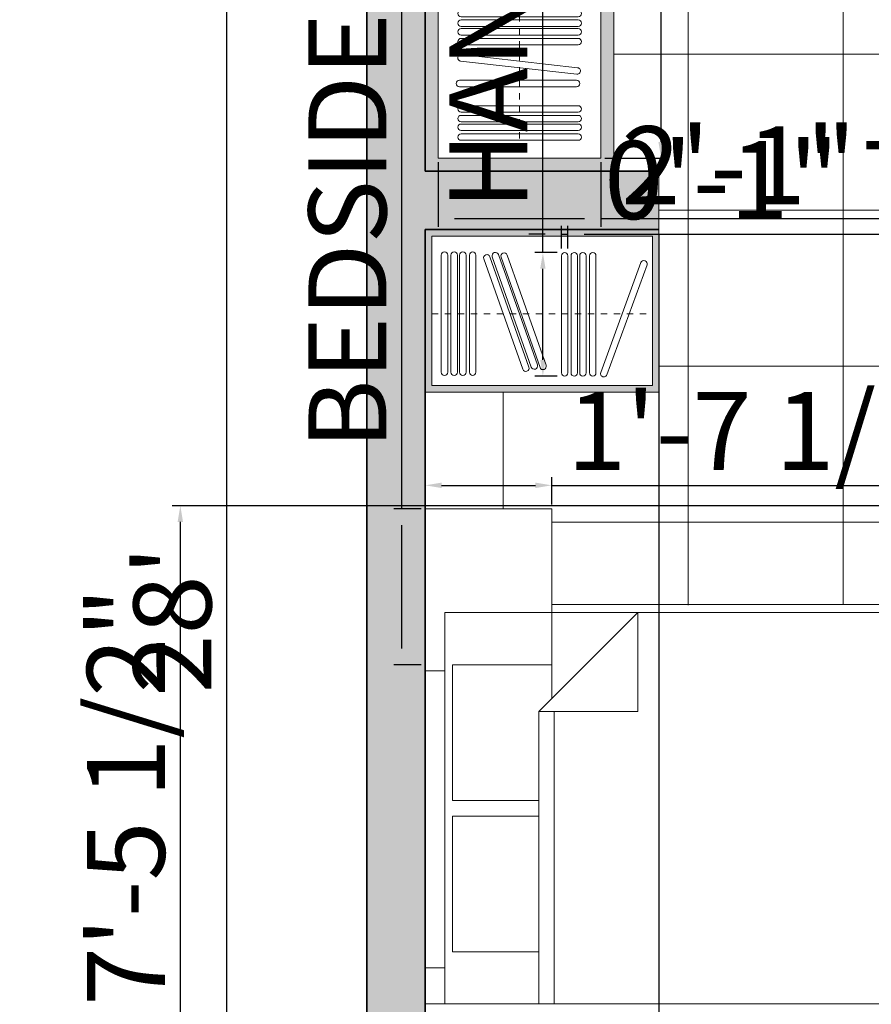
# Model space of a CAD drawing. Units: millimetres. Extents: x 542930 to 543750, y 628093 to 628738.
# Tile 3 of 14: x 542930 to 543061, y 628363 to 628514. Entities that reach past the tile are written whole.
import ezdxf

# ---------------------------------------------------------------- set-up
doc = ezdxf.new("R2010")
doc.units = ezdxf.units.MM
doc.linetypes.add('JIS_02_1.0', pattern=[2, 1, -1])
for name, color, linetype, lineweight in [('A-ANNO-DIMS', 2, 'Continuous', 18), ('A-FURN', 8, 'Continuous', 18), ('A-FURN-MILL', 8, 'Continuous', 18), ('A-FURN-MILL-HIDN', 8, 'JIS_02_1.0', 13), ('A-FURN-PATT', 9, 'Continuous', 13), ('A-WALL', 7, 'Continuous', 35)]:
    doc.layers.add(name, color=color, linetype=linetype, lineweight=lineweight)
doc.layers.add('A-FLOR-PATT', color=241, linetype='Continuous', lineweight=13, true_color=0xf7abae)
doc.layers.add('A-WALL-PATT', color=251, linetype='Continuous', lineweight=13, true_color=0x636466)
doc.styles.get("Standard").update_dxf_attribs({"font": 'arial.ttf'})
doc.dimstyles.new('ISO-25', dxfattribs={"dimtxt": 12, "dimasz": 2.5, "dimexe": 1.25, "dimexo": 0.625, "dimtad": 1, "dimdec": 0, "dimlunit": 3, "dimtxsty": 'Standard', "dimcen": 2.5, "dimadec": 0, "dimazin": 0, "dimtfac": 1, "dimtdec": 0, "dimtmove": 0, "dimatfit": 3, "dimfxl": 1, "dimarcsym": 0})

# ---------------------------------------------------------------- blocks, each defined once
blk = doc.blocks.new('Bed - Queen')
for p, q in [((0, -80.00003), (0, 0)), ((0, 0), (59.99999, 0)), ((59.99999, 0), (59.99999, -80.00003)), ((7.99999, -1.2), (28.79998, -1.2)), ((7.99999, -14.4), (7.99999, -1.2)), ((28.79998, -1.2), (28.79998, -14.4)), ((31.19999, -1.2), (51.99999, -1.2)), ((31.19999, -14.4), (31.19999, -1.2)), ((51.99999, -1.2), (51.99999, -16.4)), ((0, -14.4), (44.8, -14.4)), ((59.99999, -29.6), (44.8, -14.4)), ((44.8, -14.4), (44.8, -29.6)), ((51.99999, -16.4), (46.79936, -16.4)), ((44.8, -16.8), (0, -16.8)), ((44.8, -29.6), (59.99999, -29.6)), ((59.99999, -80.00003), (0, -80.00003))]:
    blk.add_line(p, q)
blk = doc.blocks.new('*D20')
at = {"layer": 'A-ANNO-DIMS', "color": 0, "lineweight": -2, "transparency": 16777216}
for p, q in [((542983.04, 628589.83), (542960.8, 628589.83)), ((542962.05, 628587.33), (542962.05, 628256.33)), ((542983.04, 628253.83), (542960.8, 628253.83))]:
    blk.add_line(p, q, dxfattribs=at)
at = {"layer": 'A-ANNO-DIMS', "color": 0, "transparency": 16777216}
for points in [[(542961.64, 628587.33), (542962.47, 628587.33), (542962.05, 628589.83)], [(542961.64, 628256.33), (542962.47, 628256.33), (542962.05, 628253.83)]]:
    blk.add_solid(points, dxfattribs=at)
at = {"layer": 'Defpoints', "color": 0, "transparency": 16777216}
for p in [(542983.67, 628589.83), (542962.05, 628253.83), (542983.67, 628253.83)]:
    blk.add_point(p, dxfattribs=at)
at = {"layer": 'A-ANNO-DIMS', "color": 0, "transparency": 16777216, "insert": (542955.3, 628421.83), "char_height": 12, "attachment_point": 5, "rotation": 90}
blk.add_mtext("28'", dxfattribs=at)
blk = doc.blocks.new('WARDROBE-DRESS-RAIL')
for p, q in [((0, 0), (0, 62)), ((0, 62), (25, 62)), ((3.52, 60.83), (21.52, 60.83)), ((25, 0), (25, 62)), ((3.52, 59.83), (21.52, 59.83)), ((3.52, 59.35), (21.52, 59.35)), ((3.52, 58.35), (21.52, 58.35)), ((3.52, 58.02), (21.52, 58.02)), ((3.52, 57.02), (21.52, 57.02)), ((3.52, 56.51), (21.52, 56.51)), ((3.52, 55.51), (21.52, 55.51)), ((3.57, 51.08), (21.23, 54.55)), ((3.76, 50.1), (21.43, 53.57)), ((3.52, 49.31), (21.52, 49.31)), ((3.52, 48.31), (21.52, 48.31)), ((3.52, 47.82), (21.52, 47.82)), ((3.52, 46.82), (21.52, 46.82)), ((3.52, 46.49), (21.52, 46.49)), ((3.52, 45.49), (21.52, 45.49)), ((3.57, 41.35), (21.23, 44.82)), ((3.57, 39.47), (21.23, 42.94)), ((3.76, 40.37), (21.43, 43.84)), ((3.76, 38.49), (21.43, 41.96)), ((3.52, 35.91), (21.52, 35.91)), ((3.52, 34.91), (21.52, 34.91)), ((3.52, 34.43), (21.52, 34.43)), ((3.52, 33.43), (21.52, 33.43)), ((3.52, 33.1), (21.52, 33.1)), ((3.52, 32.1), (21.52, 32.1)), ((3.52, 31.59), (21.52, 31.59)), ((3.52, 30.59), (21.52, 30.59)), ((3.27, 26.51), (21.27, 26.51)), ((3.27, 25.51), (21.27, 25.51)), ((3.52, 22.74), (21.52, 22.74)), ((3.52, 21.74), (21.52, 21.74)), ((3.52, 21.26), (21.52, 21.26)), ((3.52, 20.26), (21.52, 20.26)), ((3.52, 19.93), (21.52, 19.93)), ((3.52, 18.93), (21.52, 18.93)), ((3.52, 18.42), (21.52, 18.42)), ((3.52, 17.42), (21.52, 17.42)), ((3.56, 15.93), (21.44, 13.91)), ((3.44, 14.93), (21.33, 12.92)), ((3.27, 11.99), (21.27, 11.99)), ((3.27, 10.99), (21.27, 10.99)), ((3.52, 8.06), (21.52, 8.06)), ((3.52, 7.06), (21.52, 7.06)), ((3.52, 6.58), (21.52, 6.58)), ((3.52, 5.58), (21.52, 5.58)), ((3.52, 5.25), (21.52, 5.25)), ((3.52, 4.25), (21.52, 4.25)), ((3.52, 3.74), (21.52, 3.74)), ((3.52, 2.74), (21.52, 2.74)), ((0, 0), (25, 0))]:
    blk.add_line(p, q)
for centre, start, end in [((3.52, 60.33), 90, 270), ((21.52, 60.33), 270, 90), ((3.52, 58.85), 90, 270), ((21.52, 58.85), 270, 90), ((3.52, 57.52), 90, 270), ((21.52, 57.52), 270, 90), ((3.52, 56.01), 90, 270), ((21.52, 56.01), 270, 90), ((21.33, 54.06), 281.1082, 101.1082), ((3.67, 50.59), 101.1082, 281.1082), ((3.52, 48.81), 90, 270), ((21.52, 48.81), 270, 90), ((3.52, 47.32), 90, 270), ((21.52, 47.32), 270, 90), ((3.52, 45.99), 90, 270), ((21.52, 45.99), 270, 90), ((21.33, 44.33), 281.1082, 101.1082), ((21.33, 42.45), 281.1082, 101.1082), ((3.67, 40.86), 101.1082, 281.1082), ((3.67, 38.98), 101.1082, 281.1082), ((3.52, 35.41), 90, 270), ((21.52, 35.41), 270, 90), ((3.52, 33.93), 90, 270), ((21.52, 33.93), 270, 90), ((3.52, 32.6), 90, 270), ((21.52, 32.6), 270, 90), ((3.52, 31.09), 90, 270), ((21.52, 31.09), 270, 90), ((3.27, 26.01), 90, 270), ((21.27, 26.01), 270, 90), ((3.52, 22.24), 90, 270), ((21.52, 22.24), 270, 90), ((3.52, 20.76), 90, 270), ((21.52, 20.76), 270, 90), ((3.52, 19.43), 90, 270), ((21.52, 19.43), 270, 90), ((3.52, 17.92), 90, 270), ((21.52, 17.92), 270, 90), ((3.5, 15.43), 83.5593, 263.5593), ((21.39, 13.41), 263.5593, 83.5611), ((3.27, 11.49), 90, 270), ((21.27, 11.49), 270, 90), ((3.52, 7.56), 90, 270), ((21.52, 7.56), 270, 90), ((3.52, 6.08), 90, 270), ((21.52, 6.08), 270, 90), ((3.52, 4.75), 90, 270), ((21.52, 4.75), 270, 90), ((3.52, 3.24), 90, 270), ((21.52, 3.24), 270, 90)]:
    blk.add_arc(centre, 0.5, start, end)
blk = doc.blocks.new('WARDROBE-HANGER')
for p, q in [((0, 0.5), (0, 18.5)), ((1, 0.5), (1, 18.5))]:
    blk.add_line(p, q)
for centre, start, end in [((0.5, 18.5), 0, 180), ((0.5, 0.5), 180, 0)]:
    blk.add_arc(centre, 0.5, start, end)
blk = doc.blocks.new('BED-SIDE-STAND')
for p, q in [((19.46, 24), (0, 24)), ((19.46, 0), (19.46, 24))]:
    blk.add_line(p, q)
blk = doc.blocks.new('*D31')
at = {"layer": 'A-ANNO-DIMS', "color": 0, "lineweight": -2, "transparency": 16777216}
for p, q in [((543010.77, 628478.3), (543010.77, 628630.92)), ((543012.99, 628478.3), (543009.52, 628478.3)), ((543010.77, 628461.8), (543010.77, 628475.8)), ((543012.99, 628459.3), (543009.52, 628459.3))]:
    blk.add_line(p, q, dxfattribs=at)
at = {"layer": 'A-ANNO-DIMS', "color": 0, "transparency": 16777216}
for points in [[(543010.35, 628475.8), (543011.18, 628475.8), (543010.77, 628478.3)], [(543010.35, 628461.8), (543011.18, 628461.8), (543010.77, 628459.3)]]:
    blk.add_solid(points, dxfattribs=at)
at = {"layer": 'Defpoints', "color": 0, "transparency": 16777216}
for p in [(543010.77, 628478.3), (543013.62, 628478.3), (543013.62, 628459.3)]:
    blk.add_point(p, dxfattribs=at)
at = {"layer": 'A-ANNO-DIMS', "color": 0, "transparency": 16777216, "insert": (543003.94, 628555.86), "char_height": 12, "attachment_point": 5, "rotation": 90}
blk.add_mtext('HANGER 1\'-7" TYP.', dxfattribs=at)
blk = doc.blocks.new('*D32')
at = {"layer": 'A-ANNO-DIMS', "color": 0, "lineweight": -2, "transparency": 16777216}
for p, q in [((543011.12, 628481.15), (543008.62, 628481.15)), ((543013.62, 628478.92), (543013.62, 628482.4)), ((543013.62, 628481.15), (543014.62, 628481.15)), ((543014.62, 628478.92), (543014.62, 628482.4)), ((543017.12, 628481.15), (543094.01, 628481.15))]:
    blk.add_line(p, q, dxfattribs=at)
at = {"layer": 'A-ANNO-DIMS', "color": 0, "transparency": 16777216}
for points in [[(543011.12, 628481.56), (543011.12, 628480.73), (543013.62, 628481.15)], [(543017.12, 628481.56), (543017.12, 628480.73), (543014.62, 628481.15)]]:
    blk.add_solid(points, dxfattribs=at)
at = {"layer": 'Defpoints', "color": 0, "transparency": 16777216}
for p in [(543014.62, 628481.15), (543013.62, 628478.3), (543014.62, 628478.3)]:
    blk.add_point(p, dxfattribs=at)
at = {"layer": 'A-ANNO-DIMS', "color": 0, "transparency": 16777216, "insert": (543056.82, 628487.9), "char_height": 12, "attachment_point": 5}
blk.add_mtext('0\'-1" TYP.', dxfattribs=at)
blk = doc.blocks.new('*D43')
at = {"layer": 'A-ANNO-DIMS', "color": 0, "lineweight": -2, "transparency": 16777216}
for p, q in [((543028.97, 628554.83), (543028.97, 628735.47)), ((543020.29, 628554.83), (543030.22, 628554.83)), ((543028.97, 628495.33), (543028.97, 628552.33)), ((543020.29, 628492.83), (543030.22, 628492.83))]:
    blk.add_line(p, q, dxfattribs=at)
at = {"layer": 'A-ANNO-DIMS', "color": 0, "transparency": 16777216}
for points in [[(543028.55, 628552.33), (543029.38, 628552.33), (543028.97, 628554.83)], [(543028.55, 628495.33), (543029.38, 628495.33), (543028.97, 628492.83)]]:
    blk.add_solid(points, dxfattribs=at)
at = {"layer": 'Defpoints', "color": 0, "transparency": 16777216}
for p in [(543019.67, 628554.83), (543028.97, 628554.83), (543019.67, 628492.83)]:
    blk.add_point(p, dxfattribs=at)
at = {"layer": 'A-ANNO-DIMS', "color": 0, "transparency": 16777216, "insert": (543022.14, 628646.4), "char_height": 12, "attachment_point": 5, "rotation": 90}
blk.add_mtext('DRESS RAIL 5\'-2" TYP.', dxfattribs=at)
blk = doc.blocks.new('*D44')
at = {"layer": 'A-ANNO-DIMS', "color": 0, "lineweight": -2, "transparency": 16777216}
for p, q in [((542994.67, 628492.2), (542994.67, 628482.28)), ((543019.67, 628492.2), (543019.67, 628482.28)), ((542997.17, 628483.53), (543017.17, 628483.53)), ((543019.67, 628483.53), (543096.77, 628483.53))]:
    blk.add_line(p, q, dxfattribs=at)
at = {"layer": 'A-ANNO-DIMS', "color": 0, "transparency": 16777216}
for points in [[(542997.17, 628483.94), (542997.17, 628483.11), (542994.67, 628483.53)], [(543017.17, 628483.94), (543017.17, 628483.11), (543019.67, 628483.53)]]:
    blk.add_solid(points, dxfattribs=at)
at = {"layer": 'Defpoints', "color": 0, "transparency": 16777216}
for p in [(542994.67, 628492.83), (543019.67, 628492.83), (543019.67, 628483.53)]:
    blk.add_point(p, dxfattribs=at)
at = {"layer": 'A-ANNO-DIMS', "color": 0, "transparency": 16777216, "insert": (543059.47, 628490.18), "char_height": 12, "attachment_point": 5}
blk.add_mtext('2\'-1" TYP.', dxfattribs=at)
blk = doc.blocks.new('*D59')
at = {"layer": 'A-ANNO-DIMS', "color": 0, "lineweight": -2, "transparency": 16777216}
for p, q in [((542989.07, 628438.89), (542989.07, 628654.99)), ((542992.04, 628438.89), (542987.82, 628438.89)), ((542989.07, 628417.39), (542989.07, 628436.39)), ((542992.04, 628414.89), (542987.82, 628414.89))]:
    blk.add_line(p, q, dxfattribs=at)
at = {"layer": 'A-ANNO-DIMS', "color": 0, "transparency": 16777216}
for points in [[(542988.65, 628436.39), (542989.48, 628436.39), (542989.07, 628438.89)], [(542988.65, 628417.39), (542989.48, 628417.39), (542989.07, 628414.89)]]:
    blk.add_solid(points, dxfattribs=at)
at = {"layer": 'Defpoints', "color": 0, "transparency": 16777216}
for p in [(542989.07, 628438.89), (542992.67, 628438.89), (542992.67, 628414.89)]:
    blk.add_point(p, dxfattribs=at)
at = {"layer": 'A-ANNO-DIMS', "color": 0, "transparency": 16777216, "insert": (542982.24, 628548.19), "char_height": 12, "attachment_point": 5, "rotation": 90}
blk.add_mtext('BEDSIDE STAND 2\'-0" TYP.', dxfattribs=at)
blk = doc.blocks.new('*D60')
at = {"layer": 'A-ANNO-DIMS', "color": 0, "lineweight": -2, "transparency": 16777216}
for p, q in [((542992.67, 628439.52), (542992.67, 628443.74)), ((543012.12, 628439.52), (543012.12, 628443.74)), ((542995.17, 628442.49), (543009.62, 628442.49)), ((543012.12, 628442.49), (543115.85, 628442.49))]:
    blk.add_line(p, q, dxfattribs=at)
at = {"layer": 'A-ANNO-DIMS', "color": 0, "transparency": 16777216}
for points in [[(542995.17, 628442.91), (542995.17, 628442.08), (542992.67, 628442.49)], [(543009.62, 628442.91), (543009.62, 628442.08), (543012.12, 628442.49)]]:
    blk.add_solid(points, dxfattribs=at)
at = {"layer": 'Defpoints', "color": 0, "transparency": 16777216}
for p in [(543012.12, 628442.49), (542992.67, 628438.89), (543012.12, 628438.89)]:
    blk.add_point(p, dxfattribs=at)
at = {"layer": 'A-ANNO-DIMS', "color": 0, "transparency": 16777216, "insert": (543065.24, 628449.32), "char_height": 12, "attachment_point": 5}
blk.add_mtext('1\'-7 1/2" TYP.', dxfattribs=at)
blk = doc.blocks.new('*D75')
at = {"layer": 'A-ANNO-DIMS', "color": 0, "lineweight": -2, "transparency": 16777216}
for p, q in [((543324.54, 628439.36), (542953.72, 628439.36)), ((542954.97, 628352.33), (542954.97, 628436.86)), ((543324.54, 628349.83), (542953.72, 628349.83))]:
    blk.add_line(p, q, dxfattribs=at)
at = {"layer": 'A-ANNO-DIMS', "color": 0, "transparency": 16777216}
for points in [[(542954.55, 628436.86), (542955.38, 628436.86), (542954.97, 628439.36)], [(542954.55, 628352.33), (542955.38, 628352.33), (542954.97, 628349.83)]]:
    blk.add_solid(points, dxfattribs=at)
at = {"layer": 'Defpoints', "color": 0, "transparency": 16777216}
for p in [(542954.97, 628439.36), (543325.17, 628439.36), (543325.17, 628349.83)]:
    blk.add_point(p, dxfattribs=at)
at = {"layer": 'A-ANNO-DIMS', "color": 0, "transparency": 16777216, "insert": (542948.14, 628394.6), "char_height": 12, "attachment_point": 5, "rotation": 90}
blk.add_mtext('7\'-5 1/2"', dxfattribs=at)
blk = doc.blocks.new('*D85')
at = {"layer": 'A-ANNO-DIMS', "color": 0, "lineweight": -2, "transparency": 16777216}
for p, q in [((543028.62, 628481.2), (543028.62, 628103.84)), ((543064.67, 628481.2), (543064.67, 628103.84)), ((543031.12, 628105.09), (543062.17, 628105.09))]:
    blk.add_line(p, q, dxfattribs=at)
at = {"layer": 'A-ANNO-DIMS', "color": 0, "transparency": 16777216}
for points in [[(543031.12, 628105.5), (543031.12, 628104.67), (543028.62, 628105.09)], [(543062.17, 628105.5), (543062.17, 628104.67), (543064.67, 628105.09)]]:
    blk.add_solid(points, dxfattribs=at)
at = {"layer": 'Defpoints', "color": 0, "transparency": 16777216}
for p in [(543028.62, 628481.83), (543064.67, 628481.83), (543064.67, 628105.09)]:
    blk.add_point(p, dxfattribs=at)
at = {"layer": 'A-ANNO-DIMS', "color": 0, "transparency": 16777216, "insert": (543046.65, 628111.84), "char_height": 12, "attachment_point": 5}
blk.add_mtext('3\'-0"', dxfattribs=at)

msp = doc.modelspace()

# ---------------------------------------------------------------- hatches: boundary and pattern name
at = {"layer": 'A-FURN-PATT'}
h = msp.add_hatch(color=256, dxfattribs=at)
h.dxf.hatch_style = 1
h.paths.add_polyline_path([(543021.67, 628556.83), (542992.67, 628556.83), (542992.67, 628490.83), (543021.67, 628490.83)])
h.paths.add_polyline_path([(543019.67, 628492.83), (542994.67, 628492.83), (542994.67, 628554.83), (543019.67, 628554.83)], flags=16)
h.paths.add_polyline_path([(543016.19, 628514.57), (543007.17, 628514.57), (543007.17, 628514.08), (543016.19, 628514.08, -1), (543016.19, 628513.08), (543007.17, 628513.08), (543007.17, 628512.76), (543016.19, 628512.76, -1), (543016.19, 628511.76), (543007.17, 628511.76), (543007.17, 628511.24), (543016.19, 628511.24, -1), (543016.19, 628510.24), (543007.17, 628510.24), (543007.17, 628507.74), (543016.11, 628506.73, -1.000001), (543016, 628505.74), (543007.17, 628506.74), (543007.17, 628504.81), (543015.94, 628504.81, -1), (543015.94, 628503.81), (543007.17, 628503.81), (543007.17, 628500.89), (543016.19, 628500.89, -1), (543016.19, 628499.89), (543007.17, 628499.89), (543007.17, 628499.4), (543016.19, 628499.4, -1), (543016.19, 628498.4), (543007.17, 628498.4), (543007.17, 628498.08), (543016.19, 628498.08, -1), (543016.19, 628497.08), (543007.17, 628497.08), (543007.17, 628496.56), (543016.19, 628496.56, -1), (543016.19, 628495.56), (542998.19, 628495.56, -1), (542998.19, 628496.56), (543007.17, 628496.56), (543007.17, 628497.08), (542998.19, 628497.08, -1), (542998.19, 628498.08), (543007.17, 628498.08), (543007.17, 628498.4), (542998.19, 628498.4, -1), (542998.19, 628499.4), (543007.17, 628499.4), (543007.17, 628499.89), (542998.19, 628499.89, -1), (542998.19, 628500.89), (543007.17, 628500.89), (543007.17, 628503.81), (542997.94, 628503.81, -1), (542997.94, 628504.81), (543007.17, 628504.81), (543007.17, 628506.74), (542998.11, 628507.76, -0.999984), (542998.22, 628508.75), (543007.17, 628507.74), (543007.17, 628510.24), (542998.19, 628510.24, -1), (542998.19, 628511.24), (543007.17, 628511.24), (543007.17, 628511.76), (542998.19, 628511.76, -1), (542998.19, 628512.76), (543007.17, 628512.76), (543007.17, 628513.08), (542998.19, 628513.08, -1), (542998.19, 628514.08), (543007.17, 628514.08), (543007.17, 628514.57), (542998.19, 628514.57, -1), (542998.19, 628515.57), (543007.17, 628515.57), (543007.17, 628518.34), (542997.94, 628518.34, -1), (542997.94, 628519.34), (543007.17, 628519.34), (543007.17, 628523.41), (542998.19, 628523.41, -1), (542998.19, 628524.41), (543007.17, 628524.41), (543007.17, 628524.93), (542998.19, 628524.93, -1), (542998.19, 628525.93), (543007.17, 628525.93), (543007.17, 628526.25), (542998.19, 628526.25, -1), (542998.19, 628527.25), (543007.17, 628527.25), (543007.17, 628527.74), (542998.19, 628527.74, -1), (542998.19, 628528.74), (543007.17, 628528.74), (543007.17, 628533.03), (542998.43, 628531.31, -1.000015), (542998.24, 628532.29), (543007.17, 628534.05), (543007.17, 628534.91), (542998.43, 628533.2, -1.000015), (542998.24, 628534.18), (543007.17, 628535.93), (543007.17, 628538.32), (542998.19, 628538.32, -1), (542998.19, 628539.32), (543007.17, 628539.32), (543007.17, 628539.65), (542998.19, 628539.65, -1), (542998.19, 628540.65), (543007.17, 628540.65), (543007.17, 628541.13), (542998.19, 628541.13, -1), (542998.19, 628542.13), (543007.17, 628542.13), (543007.17, 628544.64), (542998.43, 628542.93, -1.000015), (542998.24, 628543.91), (543007.17, 628545.66), (543007.17, 628548.33), (542998.19, 628548.33, -1), (542998.19, 628549.33), (543007.17, 628549.33), (543007.17, 628549.84), (542998.19, 628549.84, -1), (542998.19, 628550.84), (543007.17, 628550.84), (543007.17, 628551.17), (542998.19, 628551.17, -1), (542998.19, 628552.17), (543007.17, 628552.17), (543007.17, 628552.66), (542998.19, 628552.66, -1), (542998.19, 628553.66), (543016.19, 628553.66, -1), (543016.19, 628552.66), (543007.17, 628552.66), (543007.17, 628552.17), (543016.19, 628552.17, -1), (543016.19, 628551.17), (543007.17, 628551.17), (543007.17, 628550.84), (543016.19, 628550.84, -1), (543016.19, 628549.84), (543007.17, 628549.84), (543007.17, 628549.33), (543016.19, 628549.33, -1), (543016.19, 628548.33), (543007.17, 628548.33), (543007.17, 628545.66), (543015.9, 628547.38, -1.000014), (543016.09, 628546.4), (543007.17, 628544.64), (543007.17, 628542.13), (543016.19, 628542.13, -0.50839), (543016.67, 628541.48), (543016.67, 628540.3, -0.156536), (543016.67, 628539.99), (543016.67, 628538.97, -0.50839), (543016.19, 628538.32), (543007.17, 628538.32), (543007.17, 628535.93), (543015.9, 628537.65, -1.000014), (543016.09, 628536.67), (543007.17, 628534.91), (543007.17, 628534.05), (543015.9, 628535.76, -1.000014), (543016.09, 628534.78), (543007.17, 628533.03), (543007.17, 628528.74), (543016.19, 628528.74, -1), (543016.19, 628527.74), (543007.17, 628527.74), (543007.17, 628527.25), (543016.19, 628527.25, -1), (543016.19, 628526.25), (543007.17, 628526.25), (543007.17, 628525.93), (543016.19, 628525.93, -1), (543016.19, 628524.93), (543007.17, 628524.93), (543007.17, 628524.41), (543016.19, 628524.41, -1), (543016.19, 628523.41), (543007.17, 628523.41), (543007.17, 628519.34), (543015.94, 628519.34, -1), (543015.94, 628518.34), (543007.17, 628518.34), (543007.17, 628515.57), (543016.19, 628515.57, -1)], flags=0)
h = msp.add_hatch(color=256, dxfattribs=at)
h.dxf.hatch_style = 1
h.paths.add_polyline_path([(543028.62, 628481.83), (542992.67, 628481.83), (542992.67, 628456.83), (543028.62, 628456.83)])
h.paths.add_polyline_path([(543027.62, 628457.83), (542993.67, 628457.83), (542993.67, 628480.83), (543027.62, 628480.83)], flags=16)
h.paths.add_polyline_path([(543020.61, 628459.51, -1), (543019.67, 628459.85), (543022.97, 628468.89), (543018.94, 628468.89), (543018.94, 628459.8, -1), (543017.94, 628459.8), (543017.94, 628468.89), (543017.43, 628468.89), (543017.43, 628459.8, -1), (543016.43, 628459.8), (543016.43, 628468.89), (543016.1, 628468.89), (543016.1, 628459.8, -1), (543015.1, 628459.8), (543015.1, 628468.89), (543014.62, 628468.89), (543014.62, 628459.8, -1), (543013.62, 628459.8), (543013.62, 628468.89), (543008.46, 628468.89), (543011.26, 628460.96, -1), (543010.32, 628460.62), (543007.4, 628468.89), (543007.14, 628468.89), (543009.92, 628461.02, -1), (543008.98, 628460.69), (543006.08, 628468.89), (543005.71, 628468.89), (543008.61, 628460.69, -1.00001), (543007.67, 628460.35), (543004.65, 628468.89), (543000.46, 628468.89), (543000.46, 628459.89, -1), (542999.46, 628459.89), (542999.46, 628468.89), (542998.94, 628468.89), (542998.94, 628459.89, -1), (542997.94, 628459.89), (542997.94, 628468.89), (542997.62, 628468.89), (542997.62, 628459.89, -1), (542996.62, 628459.89), (542996.62, 628468.89), (542996.13, 628468.89), (542996.13, 628459.89, -1), (542995.13, 628459.89), (542995.13, 628477.89, -1), (542996.13, 628477.89), (542996.13, 628468.89), (542996.62, 628468.89), (542996.62, 628477.89, -1), (542997.62, 628477.89), (542997.62, 628468.89), (542997.94, 628468.89), (542997.94, 628477.89, -1), (542998.94, 628477.89), (542998.94, 628468.89), (542999.46, 628468.89), (542999.46, 628477.89, -1), (543000.46, 628477.89), (543000.46, 628468.89), (543004.65, 628468.89), (543001.67, 628477.32, -1), (543002.61, 628477.66), (543005.71, 628468.89), (543006.08, 628468.89), (543002.98, 628477.66, -0.999986), (543003.92, 628477.99), (543007.14, 628468.89), (543007.4, 628468.89), (543004.32, 628477.6, -0.99999), (543005.26, 628477.93), (543008.46, 628468.89), (543013.62, 628468.89), (543013.62, 628477.8, -1), (543014.62, 628477.8), (543014.62, 628468.89), (543015.1, 628468.89), (543015.1, 628477.8, -1), (543016.1, 628477.8), (543016.1, 628468.89), (543016.43, 628468.89), (543016.43, 628477.8, -1), (543017.43, 628477.8), (543017.43, 628468.89), (543017.94, 628468.89), (543017.94, 628477.8, -1), (543018.94, 628477.8), (543018.94, 628468.89), (543022.97, 628468.89), (543025.85, 628476.75, -1), (543026.79, 628476.41)], flags=0)
at = {"layer": 'A-WALL-PATT'}
h = msp.add_hatch(color=256, dxfattribs=at)
h.dxf.hatch_style = 1
h.paths.add_polyline_path([(542992.67, 628481.83), (543028.62, 628481.83), (543028.62, 628490.83), (542992.67, 628490.83), (542992.67, 628580.83), (543113.07, 628580.83), (543113.07, 628589.83), (542983.67, 628589.83), (542983.67, 628335.3), (542992.67, 628335.3)])

# ---------------------------------------------------------------- linework, layer by layer
at = {"layer": 'A-FLOR-PATT'}
for p, q in [((543033.13, 628424.06), (543033.13, 628556.83)), ((543056.96, 628424.17), (543056.96, 628556.83)), ((543021.67, 628508.83), (543068.67, 628508.83)), ((543028.62, 628484.83), (543064.67, 628484.83)), ((543028.62, 628460.83), (543064.67, 628460.83)), ((543004.67, 628438.89), (543004.67, 628456.83)), ((543012.12, 628436.83), (543149.17, 628436.83))]:
    msp.add_line(p, q, dxfattribs=at)
at = {"layer": 'A-FURN'}
for p, q in [((543012.12, 628424.17), (543077.27, 628424.17)), ((542995.67, 628413.97), (542992.67, 628413.97)), ((542995.67, 628413.97), (542995.67, 628368.25)), ((542995.67, 628368.25), (542992.67, 628368.25)), ((542995.67, 628362.72), (542992.67, 628362.72))]:
    msp.add_line(p, q, dxfattribs=at)
at = {"layer": 'A-FURN-MILL'}
for p, q in [((543021.67, 628490.83), (543021.67, 628580.83)), ((543028.62, 628490.83), (543028.62, 628456.83)), ((542993.67, 628480.83), (543027.62, 628480.83)), ((542993.67, 628457.83), (542993.67, 628480.83)), ((543027.62, 628480.83), (543027.62, 628457.83)), ((542992.67, 628456.83), (543028.62, 628456.83)), ((542993.67, 628457.83), (543027.62, 628457.83))]:
    msp.add_line(p, q, dxfattribs=at)
at = {"layer": 'A-FURN-MILL-HIDN'}
for p, q in [((543007.17, 628554.83), (543007.17, 628492.83)), ((542993.67, 628468.89), (543027.29, 628468.89))]:
    msp.add_line(p, q, dxfattribs=at)
at = {"layer": 'A-WALL'}
for p, q in [((542992.67, 628490.83), (542992.67, 628580.83)), ((542992.67, 628490.83), (543028.62, 628490.83)), ((542992.67, 628262.83), (542992.67, 628481.83)), ((542992.67, 628481.83), (543028.62, 628481.83))]:
    msp.add_line(p, q, dxfattribs=at)
msp.add_lwpolyline([(543499.67, 628253.83), (542983.67, 628253.83), (542983.67, 628589.83)], dxfattribs=at)

# ---------------------------------------------------------------- block references
at = {"layer": 'A-FURN'}
msp.add_blockref('BED-SIDE-STAND', (542992.67, 628414.89), dxfattribs=at)
at = {"layer": 'A-FURN', "xscale": 1.003451310197957, "yscale": 1.003451310197957, "zscale": 1.003451310197957, "rotation": 90}
msp.add_blockref('Bed - Queen', (542995.67, 628362.72), dxfattribs=at)
at = {"layer": 'A-FURN-MILL'}
for name, p in [('WARDROBE-DRESS-RAIL', (542994.67, 628492.83)), ('WARDROBE-HANGER', (542995.13, 628459.39)), ('WARDROBE-HANGER', (542996.62, 628459.39)), ('WARDROBE-HANGER', (542997.94, 628459.39)), ('WARDROBE-HANGER', (542999.46, 628459.39)), ('WARDROBE-HANGER', (543013.62, 628459.3)), ('WARDROBE-HANGER', (543015.1, 628459.3)), ('WARDROBE-HANGER', (543016.43, 628459.3)), ('WARDROBE-HANGER', (543017.94, 628459.3))]:
    msp.add_blockref(name, p, dxfattribs=at)
for p, rotation in [((543007.84, 628459.88), 19.47387642928381), ((543009.15, 628460.21), 19.47387642860089), ((543010.49, 628460.15), 19.47387642928381), ((543019.5, 628459.38), 339.9189924069234)]:
    msp.add_blockref('WARDROBE-HANGER', p, dxfattribs=dict(at, rotation=rotation))

# ---------------------------------------------------------------- dimensions: what is measured, and where the dimension line sits
at = {"layer": 'A-ANNO-DIMS'}
for base, p1, p2, text, picture, middle in [((543028.97, 628554.83), (543019.67, 628492.83), (543019.67, 628554.83), 'DRESS RAIL <> TYP.', '*D43', (543022.14, 628646.4)), ((542989.07, 628438.89), (542992.67, 628414.89), (542992.67, 628438.89), 'BEDSIDE STAND <> TYP.', '*D59', (542982.24, 628548.19)), ((543010.77, 628478.3), (543013.62, 628459.3), (543013.62, 628478.3), 'HANGER <> TYP.', '*D31', (543003.94, 628555.86))]:
    dim = msp.add_linear_dim(base=base, p1=p1, p2=p2, angle=90, text=text, dimstyle='ISO-25', override={"dimdec": 1, "dimlfac": 1, "dimrnd": 0, "dimzin": 1, "dimdsep": 46, "dimlunit": 4, "dimfrac": 2}, dxfattribs=at)
    dim.commit()
    dim.dimension.update_dxf_attribs({"geometry": picture, "text_midpoint": middle})
for base, p1, p2, override, picture, middle in [((542962.05, 628253.83), (542983.67, 628589.83), (542983.67, 628253.83), {"dimclrd": 0, "dimclre": 0, "dimclrt": 0}, '*D20', (542955.3, 628421.83)), ((542954.97, 628439.36), (543325.17, 628349.83), (543325.17, 628439.36), {"dimdec": 1, "dimlfac": 1, "dimrnd": 0, "dimzin": 1, "dimdsep": 46, "dimlunit": 4, "dimfrac": 2}, '*D75', (542948.14, 628394.6))]:
    dim = msp.add_linear_dim(base=base, p1=p1, p2=p2, angle=90, dimstyle='ISO-25', override=override, dxfattribs=at)
    dim.commit()
    dim.dimension.update_dxf_attribs({"geometry": picture, "text_midpoint": middle})
for base, p1, p2, picture, middle in [((543019.67, 628483.53), (542994.67, 628492.83), (543019.67, 628492.83), '*D44', (543059.47, 628490.18)), ((543014.62, 628481.15), (543013.62, 628478.3), (543014.62, 628478.3), '*D32', (543056.82, 628487.9)), ((543012.1235, 628442.4945), (542992.6669, 628438.8945), (543012.1235, 628438.8945), '*D60', (543065.2376, 628449.3241))]:
    dim = msp.add_linear_dim(base=base, p1=p1, p2=p2, text='<> TYP.', dimstyle='ISO-25', override={"dimdec": 1, "dimlfac": 1, "dimrnd": 0, "dimzin": 1, "dimdsep": 46, "dimlunit": 4, "dimfrac": 2}, dxfattribs=at)
    dim.commit()
    dim.dimension.update_dxf_attribs({"geometry": picture, "text_midpoint": middle})
dim = msp.add_linear_dim(base=(543064.6669, 628105.0858), p1=(543028.6237, 628481.8258), p2=(543064.6669, 628481.8258), dimstyle='ISO-25', override={"dimdec": 1, "dimlfac": 1, "dimrnd": 0, "dimzin": 1, "dimdsep": 46, "dimlunit": 4, "dimfrac": 2}, dxfattribs=at)
dim.commit()
dim.dimension.update_dxf_attribs({"geometry": '*D85', "text_midpoint": (543046.6453, 628111.8418)})

doc.saveas('drawing.dxf')
